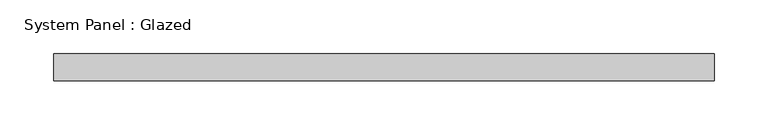
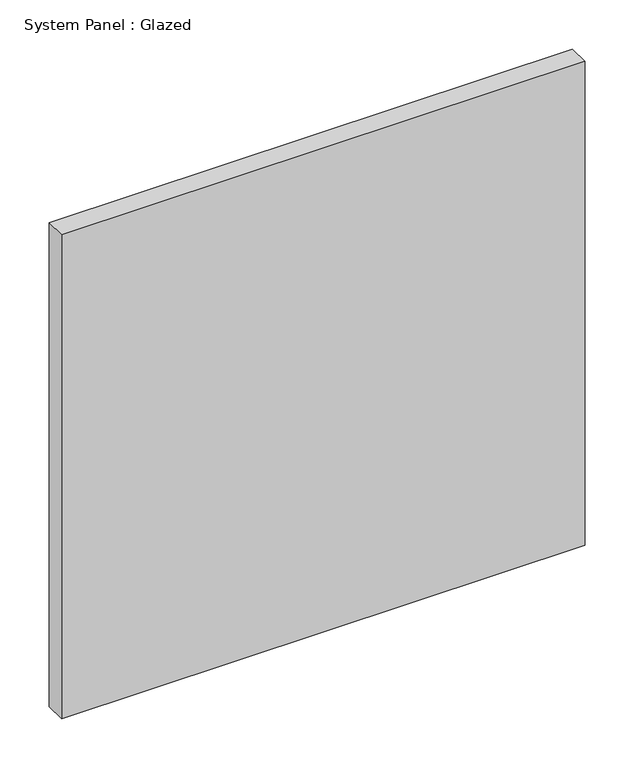
"""IFC4 building model written with IfcOpenShell, lengths in millimetres: plate geometry, System Panel : Glazed."""

from ifc_helpers import new_model, si_unit, origin, origin_with_axes, place, context, project, spatial, polyline, outline, extrude, source, transform, mapped, element, save


def system_panel_glazed_23e43b4f(model_context):
    return source(origin(), model_context, "Body", "SweptSolid", [
        extrude(outline(polyline([(307.975, 19.05), (-307.975, 19.05), (-307.975, 44.45), (307.975, 44.45), (307.975, 19.05)])), origin_with_axes(), (0.0, 0.0, 1.0), 601.6943895),
    ])


if __name__ == "__main__":
    model = new_model("IFC4")
    model_context = context("Model", 3, world=origin())
    ifc_project = project(units=[si_unit("LENGTHUNIT", "METRE", prefix="MILLI")], contexts=[model_context])
    site = spatial("IfcSite", under=ifc_project)
    building = spatial("IfcBuilding", under=site)
    placement = place(None, origin())
    system_panel_glazed_shape = system_panel_glazed_23e43b4f(model_context)
    element("IfcPlate", 1, ObjectType="System Panel : Glazed", at=placement, inside=building, context=model_context, shape_type="MappedRepresentation", body=[
        mapped(system_panel_glazed_shape, transform((0.0, 0.0, 0.0), x_axis=(1.0, 0.0, 0.0), y_axis=(0.0, 1.0, 0.0), z_axis=(0.0, 0.0, 1.0))),
    ])
    save(model, "model.ifc")

# Revit data of these elements
# Type "System Panel : Glazed"
#   Construction Type Id = "GSP4R"
#   Analytic Construction = "1/8 in Pilkington single glazing"
#   Visual Light Transmittance = 0.9
#   Solar Heat Gain Coefficient = 0.86
#   Heat Transfer Coefficient (U) = 1.18115 BTU/(h·ft²·°F)
#   Define Thermal Properties by = 1
# Element 1 (IfcPlate, "System Panel : Glazed")
#   Materials on its faces: "Glass"
# Materials
#   "Glass": class "Glass", colour RGB 0 128 192, transparency 0.75, Description = "Soda Lime Glass", Cost = 0
